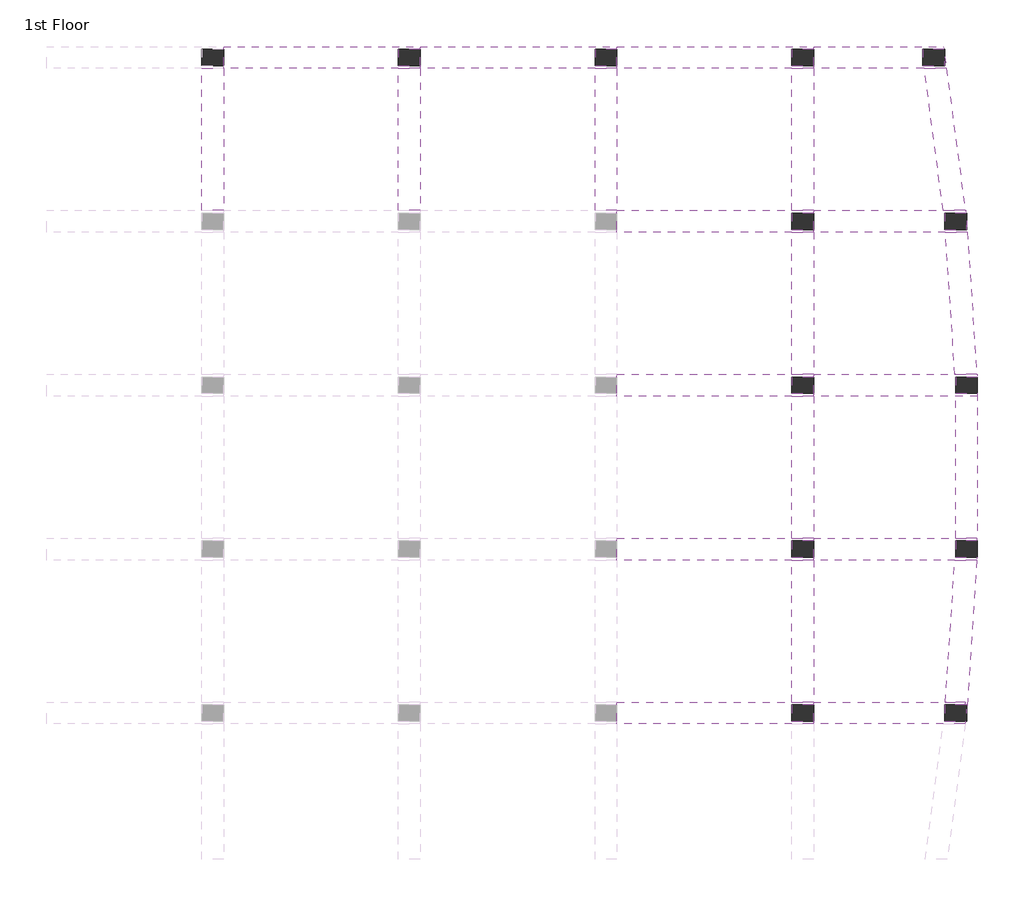
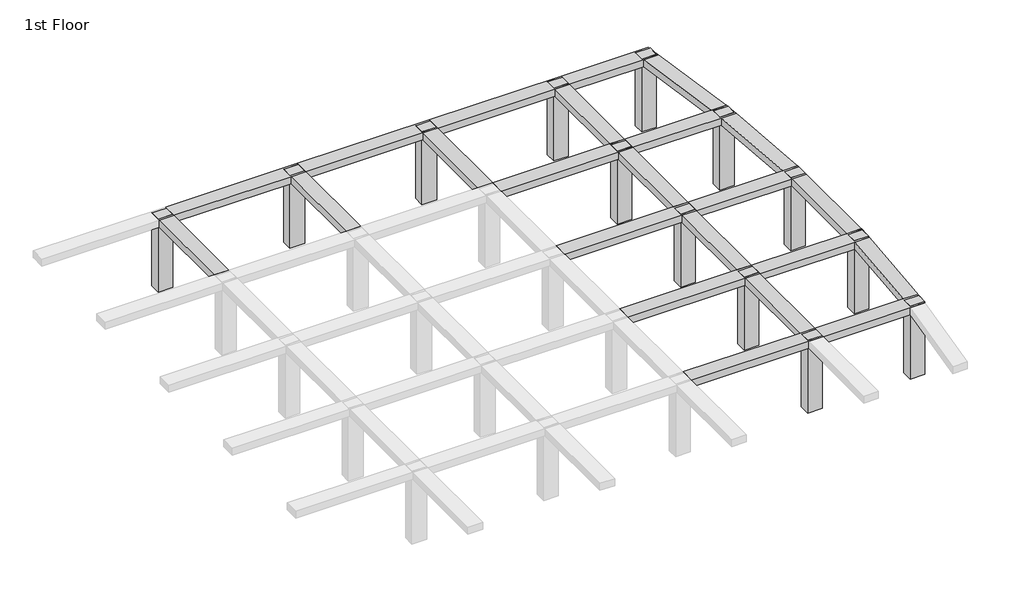
# One storey, part 3 of 3: 23 beams, 13 columns.
"""IFC4 building model written with IfcOpenShell, lengths in millimetres."""

from ifc_helpers import new_model, si_unit, frame, origin, place, context, project, spatial, polyline, outline, extrude, faceted_brep, element, save

model = new_model("IFC4")

# Units and contexts
model_context = context("Model", 3, world=origin())
ifc_project = project(units=[si_unit("LENGTHUNIT", "METRE", prefix="MILLI")], contexts=[model_context])

# Site, building, storey
site = spatial("IfcSite", under=ifc_project)
building = spatial("IfcBuilding", under=site)
storey = spatial("IfcBuildingStorey", under=building, Name="1st Floor", Elevation=3200.4)

# Beams
placement = place(None, origin())
element("IfcBeam", 1, ObjectType="Concrete-Rectangular Beam : 2' x2'", at=placement, inside=storey, context=model_context, shape_type="Brep", body=[
    faceted_brep([(-160.074232, 1680.7831222, 6400.8), (-160.074232, 1604.5831222, 6400.8), (-160.074232, 1147.3831222, 6400.8), (-160.074232, 1071.1831222, 6400.8), (4716.725768, 1071.1831222, 6400.8), (5326.325768, 1071.1831222, 6400.8), (5326.325768, 1147.3831222, 6400.8), (4716.725768, 1147.3831222, 6400.8), (4716.725768, 1604.5831222, 6400.8), (5326.325768, 1604.5831222, 6400.8), (5326.325768, 1680.7831222, 6400.8), (4716.725768, 1680.7831222, 6400.8), (-160.074232, 1071.1831222, 6096.0), (4716.725768, 1071.1831222, 6096.0), (5326.325768, 1071.1831222, 6096.0), (-160.074232, 1147.3831222, 6096.0), (-160.074232, 1604.5831222, 6096.0), (-160.074232, 1680.7831222, 6096.0), (4716.725768, 1680.7831222, 6096.0), (5326.325768, 1680.7831222, 6096.0), (5326.325768, 1604.5831222, 6096.0), (4716.725768, 1604.5831222, 6096.0), (4716.725768, 1147.3831222, 6096.0), (5326.325768, 1147.3831222, 6096.0)], [[[0, 1, 2, 3, 4, 5, 6, 7, 8, 9, 10, 11]], [[3, 12, 13, 14, 5, 4]], [[12, 15, 16, 17, 18, 19, 20, 21, 22, 23, 14, 13]], [[10, 19, 18, 17, 0, 11]], [[3, 2, 1, 0, 17, 16, 15, 12]], [[5, 14, 23, 6]], [[22, 7, 6, 23]], [[7, 22, 21, 8]], [[8, 21, 20, 9]], [[19, 10, 9, 20]]]),
])
element("IfcBeam", 2, ObjectType="Concrete-Rectangular Beam : 2' x2'", at=placement, inside=storey, context=model_context, shape_type="Brep", body=[
    faceted_brep([(9555.2251658, 1680.7831222, 6400.8), (9003.0522312, 1680.7831222, 6400.8), (5326.325768, 1680.7831222, 6400.8), (5326.325768, 1604.5831222, 6400.8), (5326.325768, 1147.3831222, 6400.8), (5326.325768, 1071.1831222, 6400.8), (8940.2370643, 1071.1831222, 6400.8), (9555.2251658, 1071.1831222, 6400.8), (9555.2251658, 1147.3831222, 6400.8), (8983.5457827, 1147.3831222, 6400.8), (8983.5457827, 1604.5831222, 6400.8), (9555.2251658, 1604.5831222, 6400.8), (9555.2251658, 1071.1831222, 6096.0), (5326.325768, 1071.1831222, 6096.0), (8940.2370643, 1071.1831222, 6096.0), (5326.325768, 1147.3831222, 6096.0), (5326.325768, 1604.5831222, 6096.0), (5326.325768, 1680.7831222, 6096.0), (9003.0522312, 1680.7831222, 6096.0), (9555.2251658, 1680.7831222, 6096.0), (9555.2251658, 1604.5831222, 6096.0), (8983.5457827, 1604.5831222, 6096.0), (8983.5457827, 1147.3831222, 6096.0), (9555.2251658, 1147.3831222, 6096.0)], [[[0, 1, 2, 3, 4, 5, 6, 7, 8, 9, 10, 11]], [[12, 7, 6, 5, 13, 14]], [[12, 14, 13, 15, 16, 17, 18, 19, 20, 21, 22, 23]], [[0, 19, 18, 17, 2, 1]], [[7, 12, 23, 8]], [[5, 4, 3, 2, 17, 16, 15, 13]], [[22, 9, 8, 23]], [[9, 22, 21, 10]], [[10, 21, 20, 11]], [[19, 0, 11, 20]]]),
])
element("IfcBeam", 3, ObjectType="Concrete-Rectangular Beam : 2' x2'", at=placement, inside=storey, context=model_context, shape_type="Brep", body=[
    faceted_brep([(-160.074232, 6252.7831222, 6400.8), (-160.074232, 6176.5831222, 6400.8), (-160.074232, 5719.3831222, 6400.8), (-160.074232, 5643.1831222, 6400.8), (4716.725768, 5643.1831222, 6400.8), (5326.325768, 5643.1831222, 6400.8), (5326.325768, 5719.3831222, 6400.8), (4716.725768, 5719.3831222, 6400.8), (4716.725768, 6176.5831222, 6400.8), (5326.325768, 6176.5831222, 6400.8), (5326.325768, 6252.7831222, 6400.8), (4716.725768, 6252.7831222, 6400.8), (-160.074232, 5643.1831222, 6096.0), (4716.725768, 5643.1831222, 6096.0), (5326.325768, 5643.1831222, 6096.0), (-160.074232, 5719.3831222, 6096.0), (-160.074232, 6176.5831222, 6096.0), (-160.074232, 6252.7831222, 6096.0), (4716.725768, 6252.7831222, 6096.0), (5326.325768, 6252.7831222, 6096.0), (5326.325768, 6176.5831222, 6096.0), (4716.725768, 6176.5831222, 6096.0), (4716.725768, 5719.3831222, 6096.0), (5326.325768, 5719.3831222, 6096.0)], [[[0, 1, 2, 3, 4, 5, 6, 7, 8, 9, 10, 11]], [[3, 12, 13, 14, 5, 4]], [[12, 15, 16, 17, 18, 19, 20, 21, 22, 23, 14, 13]], [[10, 19, 18, 17, 0, 11]], [[3, 2, 1, 0, 17, 16, 15, 12]], [[5, 14, 23, 6]], [[22, 7, 6, 23]], [[7, 22, 21, 8]], [[8, 21, 20, 9]], [[19, 10, 9, 20]]]),
])
element("IfcBeam", 4, ObjectType="Concrete-Rectangular Beam : 2' x2'", at=placement, inside=storey, context=model_context, shape_type="Brep", body=[
    faceted_brep([(9876.2389574, 6252.7831222, 6400.8), (9286.1454059, 6252.7831222, 6400.8), (5326.325768, 6252.7831222, 6400.8), (5326.325768, 6176.5831222, 6400.8), (5326.325768, 5719.3831222, 6400.8), (5326.325768, 5643.1831222, 6400.8), (9265.305238, 5643.1831222, 6400.8), (9876.2389574, 5643.1831222, 6400.8), (9876.2389574, 5719.3831222, 6400.8), (9286.1454059, 5719.3831222, 6400.8), (9286.1454059, 6176.5831222, 6400.8), (9876.2389574, 6176.5831222, 6400.8), (9876.2389574, 5643.1831222, 6096.0), (5326.325768, 5643.1831222, 6096.0), (9265.305238, 5643.1831222, 6096.0), (5326.325768, 5719.3831222, 6096.0), (5326.325768, 6176.5831222, 6096.0), (5326.325768, 6252.7831222, 6096.0), (9286.1454059, 6252.7831222, 6096.0), (9876.2389574, 6252.7831222, 6096.0), (9876.2389574, 6176.5831222, 6096.0), (9286.1454059, 6176.5831222, 6096.0), (9286.1454059, 5719.3831222, 6096.0), (9876.2389574, 5719.3831222, 6096.0)], [[[0, 1, 2, 3, 4, 5, 6, 7, 8, 9, 10, 11]], [[12, 7, 6, 5, 13, 14]], [[12, 14, 13, 15, 16, 17, 18, 19, 20, 21, 22, 23]], [[0, 19, 18, 17, 2, 1]], [[7, 12, 23, 8]], [[5, 4, 3, 2, 17, 16, 15, 13]], [[22, 9, 8, 23]], [[9, 22, 21, 10]], [[10, 21, 20, 11]], [[19, 0, 11, 20]]]),
])
element("IfcBeam", 5, ObjectType="Concrete-Rectangular Beam : 2' x2'", at=placement, inside=storey, context=model_context, shape_type="Brep", body=[
    faceted_brep([(-160.074232, 10824.7831222, 6400.8), (-160.074232, 10748.5831222, 6400.8), (-160.074232, 10291.3831222, 6400.8), (-160.074232, 10215.1831222, 6400.8), (4716.725768, 10215.1831222, 6400.8), (5326.325768, 10215.1831222, 6400.8), (5326.325768, 10291.3831222, 6400.8), (4716.725768, 10291.3831222, 6400.8), (4716.725768, 10748.5831222, 6400.8), (5326.325768, 10748.5831222, 6400.8), (5326.325768, 10824.7831222, 6400.8), (4716.725768, 10824.7831222, 6400.8), (-160.074232, 10215.1831222, 6096.0), (4716.725768, 10215.1831222, 6096.0), (5326.325768, 10215.1831222, 6096.0), (-160.074232, 10291.3831222, 6096.0), (-160.074232, 10748.5831222, 6096.0), (-160.074232, 10824.7831222, 6096.0), (4716.725768, 10824.7831222, 6096.0), (5326.325768, 10824.7831222, 6096.0), (5326.325768, 10748.5831222, 6096.0), (4716.725768, 10748.5831222, 6096.0), (4716.725768, 10291.3831222, 6096.0), (5326.325768, 10291.3831222, 6096.0)], [[[0, 1, 2, 3, 4, 5, 6, 7, 8, 9, 10, 11]], [[3, 12, 13, 14, 5, 4]], [[12, 15, 16, 17, 18, 19, 20, 21, 22, 23, 14, 13]], [[10, 19, 18, 17, 0, 11]], [[3, 2, 1, 0, 17, 16, 15, 12]], [[5, 14, 23, 6]], [[22, 7, 6, 23]], [[7, 22, 21, 8]], [[8, 21, 20, 9]], [[19, 10, 9, 20]]]),
])
element("IfcBeam", 6, ObjectType="Concrete-Rectangular Beam : 2' x2'", at=placement, inside=storey, context=model_context, shape_type="Brep", body=[
    faceted_brep([(9895.7454059, 10824.7831222, 6400.8), (9876.2389574, 10824.7831222, 6400.8), (9265.305238, 10824.7831222, 6400.8), (5326.325768, 10824.7831222, 6400.8), (5326.325768, 10748.5831222, 6400.8), (5326.325768, 10291.3831222, 6400.8), (5326.325768, 10215.1831222, 6400.8), (9895.7454059, 10215.1831222, 6400.8), (9895.7454059, 10291.3831222, 6400.8), (9286.1454059, 10291.3831222, 6400.8), (9286.1454059, 10748.5831222, 6400.8), (9895.7454059, 10748.5831222, 6400.8), (9895.7454059, 10215.1831222, 6096.0), (5326.325768, 10215.1831222, 6096.0), (5326.325768, 10291.3831222, 6096.0), (5326.325768, 10748.5831222, 6096.0), (5326.325768, 10824.7831222, 6096.0), (9265.305238, 10824.7831222, 6096.0), (9876.2389574, 10824.7831222, 6096.0), (9895.7454059, 10824.7831222, 6096.0), (9895.7454059, 10748.5831222, 6096.0), (9286.1454059, 10748.5831222, 6096.0), (9286.1454059, 10291.3831222, 6096.0), (9895.7454059, 10291.3831222, 6096.0)], [[[0, 1, 2, 3, 4, 5, 6, 7, 8, 9, 10, 11]], [[12, 7, 6, 13]], [[12, 13, 14, 15, 16, 17, 18, 19, 20, 21, 22, 23]], [[0, 19, 18, 17, 16, 3, 2, 1]], [[7, 12, 23, 8]], [[6, 5, 4, 3, 16, 15, 14, 13]], [[22, 9, 8, 23]], [[9, 22, 21, 10]], [[10, 21, 20, 11]], [[19, 0, 11, 20]]]),
])
element("IfcBeam", 7, ObjectType="Concrete-Rectangular Beam : 2' x2'", at=placement, inside=storey, context=model_context, shape_type="Brep", body=[
    faceted_brep([(-160.074232, 15396.7831222, 6400.8), (-160.074232, 15320.5831222, 6400.8), (-160.074232, 14863.3831222, 6400.8), (-160.074232, 14787.1831222, 6400.8), (4716.725768, 14787.1831222, 6400.8), (5326.325768, 14787.1831222, 6400.8), (5326.325768, 14863.3831222, 6400.8), (4716.725768, 14863.3831222, 6400.8), (4716.725768, 15320.5831222, 6400.8), (5326.325768, 15320.5831222, 6400.8), (5326.325768, 15396.7831222, 6400.8), (4716.725768, 15396.7831222, 6400.8), (-160.074232, 14787.1831222, 6096.0), (4716.725768, 14787.1831222, 6096.0), (5326.325768, 14787.1831222, 6096.0), (-160.074232, 14863.3831222, 6096.0), (-160.074232, 15320.5831222, 6096.0), (-160.074232, 15396.7831222, 6096.0), (4716.725768, 15396.7831222, 6096.0), (5326.325768, 15396.7831222, 6096.0), (5326.325768, 15320.5831222, 6096.0), (4716.725768, 15320.5831222, 6096.0), (4716.725768, 14863.3831222, 6096.0), (5326.325768, 14863.3831222, 6096.0)], [[[0, 1, 2, 3, 4, 5, 6, 7, 8, 9, 10, 11]], [[3, 12, 13, 14, 5, 4]], [[12, 15, 16, 17, 18, 19, 20, 21, 22, 23, 14, 13]], [[10, 19, 18, 17, 0, 11]], [[3, 2, 1, 0, 17, 16, 15, 12]], [[5, 14, 23, 6]], [[22, 7, 6, 23]], [[7, 22, 21, 8]], [[8, 21, 20, 9]], [[19, 10, 9, 20]]]),
])
element("IfcBeam", 8, ObjectType="Concrete-Rectangular Beam : 2' x2'", at=placement, inside=storey, context=model_context, shape_type="Brep", body=[
    faceted_brep([(9573.6393342, 15396.7831222, 6400.8), (9555.2251658, 15396.7831222, 6400.8), (8940.2370643, 15396.7831222, 6400.8), (5326.325768, 15396.7831222, 6400.8), (5326.325768, 15320.5831222, 6400.8), (5326.325768, 14863.3831222, 6400.8), (5326.325768, 14787.1831222, 6400.8), (9003.0522312, 14787.1831222, 6400.8), (9613.9859506, 14787.1831222, 6400.8), (9593.1457827, 15102.0587543, 6400.8), (9593.1457827, 14863.3831222, 6400.8), (8983.5457827, 14863.3831222, 6400.8), (8983.5457827, 15320.5831222, 6400.8), (9578.6826612, 15320.5831222, 6400.8), (9613.9859506, 14787.1831222, 6096.0), (5326.325768, 14787.1831222, 6096.0), (9003.0522312, 14787.1831222, 6096.0), (5326.325768, 14863.3831222, 6096.0), (5326.325768, 15320.5831222, 6096.0), (5326.325768, 15396.7831222, 6096.0), (8940.2370643, 15396.7831222, 6096.0), (9555.2251658, 15396.7831222, 6096.0), (9573.6393342, 15396.7831222, 6096.0), (9578.6826612, 15320.5831222, 6096.0), (8983.5457827, 15320.5831222, 6096.0), (8983.5457827, 14863.3831222, 6096.0), (9593.1457827, 14863.3831222, 6096.0), (9593.1457827, 15102.0587543, 6096.0)], [[[0, 1, 2, 3, 4, 5, 6, 7, 8, 9, 10, 11, 12, 13]], [[14, 8, 7, 6, 15, 16]], [[14, 16, 15, 17, 18, 19, 20, 21, 22, 23, 24, 25, 26, 27]], [[0, 22, 21, 20, 19, 3, 2, 1]], [[8, 14, 27, 9]], [[6, 5, 4, 3, 19, 18, 17, 15]], [[26, 10, 9, 27]], [[10, 26, 25, 11]], [[11, 25, 24, 12]], [[12, 24, 23, 13]], [[22, 0, 13, 23]]]),
])
element("IfcBeam", 9, ObjectType="Concrete-Rectangular Beam : 2' x2'", at=placement, inside=storey, context=model_context, shape_type="Brep", body=[
    faceted_brep([(-11132.874232, 19968.7831222, 6400.8), (-11132.874232, 19892.5831222, 6400.8), (-11132.874232, 19435.3831222, 6400.8), (-11132.874232, 19359.1831222, 6400.8), (-6256.074232, 19359.1831222, 6400.8), (-5646.474232, 19359.1831222, 6400.8), (-5646.474232, 19435.3831222, 6400.8), (-6256.074232, 19435.3831222, 6400.8), (-6256.074232, 19892.5831222, 6400.8), (-5646.474232, 19892.5831222, 6400.8), (-5646.474232, 19968.7831222, 6400.8), (-11132.874232, 19359.1831222, 6096.0), (-6256.074232, 19359.1831222, 6096.0), (-5646.474232, 19359.1831222, 6096.0), (-11132.874232, 19435.3831222, 6096.0), (-11132.874232, 19892.5831222, 6096.0), (-11132.874232, 19968.7831222, 6096.0), (-5646.474232, 19968.7831222, 6096.0), (-5646.474232, 19892.5831222, 6096.0), (-6256.074232, 19892.5831222, 6096.0), (-6256.074232, 19435.3831222, 6096.0), (-5646.474232, 19435.3831222, 6096.0)], [[[0, 1, 2, 3, 4, 5, 6, 7, 8, 9, 10]], [[3, 11, 12, 13, 5, 4]], [[11, 14, 15, 16, 17, 18, 19, 20, 21, 13, 12]], [[10, 17, 16, 0]], [[3, 2, 1, 0, 16, 15, 14, 11]], [[5, 13, 21, 6]], [[20, 7, 6, 21]], [[7, 20, 19, 8]], [[8, 19, 18, 9]], [[17, 10, 9, 18]]]),
])
element("IfcBeam", 10, ObjectType="Concrete-Rectangular Beam : 2' x2'", at=placement, inside=storey, context=model_context, shape_type="Brep", body=[
    faceted_brep([(-160.074232, 19968.7831222, 6400.8), (-5646.474232, 19968.7831222, 6400.8), (-5646.474232, 19892.5831222, 6400.8), (-5646.474232, 19435.3831222, 6400.8), (-5646.474232, 19359.1831222, 6400.8), (-769.674232, 19359.1831222, 6400.8), (-160.074232, 19359.1831222, 6400.8), (-160.074232, 19435.3831222, 6400.8), (-769.674232, 19435.3831222, 6400.8), (-769.674232, 19892.5831222, 6400.8), (-160.074232, 19892.5831222, 6400.8), (-160.074232, 19359.1831222, 6096.0), (-5646.474232, 19359.1831222, 6096.0), (-769.674232, 19359.1831222, 6096.0), (-5646.474232, 19435.3831222, 6096.0), (-5646.474232, 19892.5831222, 6096.0), (-5646.474232, 19968.7831222, 6096.0), (-160.074232, 19968.7831222, 6096.0), (-160.074232, 19892.5831222, 6096.0), (-769.674232, 19892.5831222, 6096.0), (-769.674232, 19435.3831222, 6096.0), (-160.074232, 19435.3831222, 6096.0)], [[[0, 1, 2, 3, 4, 5, 6, 7, 8, 9, 10]], [[11, 6, 5, 4, 12, 13]], [[11, 13, 12, 14, 15, 16, 17, 18, 19, 20, 21]], [[0, 17, 16, 1]], [[6, 11, 21, 7]], [[4, 3, 2, 1, 16, 15, 14, 12]], [[20, 8, 7, 21]], [[8, 20, 19, 9]], [[9, 19, 18, 10]], [[17, 0, 10, 18]]]),
])
element("IfcBeam", 11, ObjectType="Concrete-Rectangular Beam : 2' x2'", at=placement, inside=storey, context=model_context, shape_type="Brep", body=[
    faceted_brep([(-160.074232, 19968.7831222, 6400.8), (-160.074232, 19892.5831222, 6400.8), (-160.074232, 19435.3831222, 6400.8), (-160.074232, 19359.1831222, 6400.8), (4716.725768, 19359.1831222, 6400.8), (5326.325768, 19359.1831222, 6400.8), (5326.325768, 19435.3831222, 6400.8), (4716.725768, 19435.3831222, 6400.8), (4716.725768, 19892.5831222, 6400.8), (5326.325768, 19892.5831222, 6400.8), (5326.325768, 19968.7831222, 6400.8), (-160.074232, 19359.1831222, 6096.0), (4716.725768, 19359.1831222, 6096.0), (5326.325768, 19359.1831222, 6096.0), (-160.074232, 19435.3831222, 6096.0), (-160.074232, 19892.5831222, 6096.0), (-160.074232, 19968.7831222, 6096.0), (5326.325768, 19968.7831222, 6096.0), (5326.325768, 19892.5831222, 6096.0), (4716.725768, 19892.5831222, 6096.0), (4716.725768, 19435.3831222, 6096.0), (5326.325768, 19435.3831222, 6096.0)], [[[0, 1, 2, 3, 4, 5, 6, 7, 8, 9, 10]], [[3, 11, 12, 13, 5, 4]], [[11, 14, 15, 16, 17, 18, 19, 20, 21, 13, 12]], [[10, 17, 16, 0]], [[3, 2, 1, 0, 16, 15, 14, 11]], [[5, 13, 21, 6]], [[20, 7, 6, 21]], [[7, 20, 19, 8]], [[8, 19, 18, 9]], [[17, 10, 9, 18]]]),
])
element("IfcBeam", 12, ObjectType="Concrete-Rectangular Beam : 2' x2'", at=placement, inside=storey, context=model_context, shape_type="Brep", body=[
    faceted_brep([(5326.325768, 19968.7831222, 6400.8), (5326.325768, 19892.5831222, 6400.8), (5326.325768, 19435.3831222, 6400.8), (5326.325768, 19359.1831222, 6400.8), (8412.2463849, 19359.1831222, 6400.8), (9027.2344863, 19359.1831222, 6400.8), (8983.925768, 19684.2011052, 6400.8), (8983.925768, 19435.3831222, 6400.8), (8374.325768, 19435.3831222, 6400.8), (8374.325768, 19892.5831222, 6400.8), (8956.158818, 19892.5831222, 6400.8), (8946.005151, 19968.7831222, 6400.8), (5326.325768, 19359.1831222, 6096.0), (8412.2463849, 19359.1831222, 6096.0), (9027.2344863, 19359.1831222, 6096.0), (5326.325768, 19435.3831222, 6096.0), (5326.325768, 19892.5831222, 6096.0), (5326.325768, 19968.7831222, 6096.0), (8946.005151, 19968.7831222, 6096.0), (8956.158818, 19892.5831222, 6096.0), (8374.325768, 19892.5831222, 6096.0), (8374.325768, 19435.3831222, 6096.0), (8983.925768, 19435.3831222, 6096.0), (8983.925768, 19684.2011052, 6096.0)], [[[0, 1, 2, 3, 4, 5, 6, 7, 8, 9, 10, 11]], [[3, 12, 13, 14, 5, 4]], [[12, 15, 16, 17, 18, 19, 20, 21, 22, 23, 14, 13]], [[11, 18, 17, 0]], [[3, 2, 1, 0, 17, 16, 15, 12]], [[5, 14, 23, 6]], [[22, 7, 6, 23]], [[7, 22, 21, 8]], [[8, 21, 20, 9]], [[9, 20, 19, 10]], [[18, 11, 10, 19]]]),
])
element("IfcBeam", 13, ObjectType="Concrete-Rectangular Beam : 2' x2'", at=placement, inside=storey, context=model_context, shape_type="SweptSolid", body=[
    extrude(outline(polyline([(-11132.874232, 15396.7831222), (-11742.474232, 15396.7831222), (-11742.474232, 19359.1831222), (-11132.874232, 19359.1831222), (-11132.874232, 15396.7831222)])), frame((0.0, 0.0, 6096.0), z_axis=(0.0, 0.0, 1.0), x_axis=(1.0, 0.0, 0.0)), (0.0, 0.0, 1.0), 304.8),
])
element("IfcBeam", 14, ObjectType="Concrete-Rectangular Beam : 2' x2'", at=placement, inside=storey, context=model_context, shape_type="SweptSolid", body=[
    extrude(outline(polyline([(-5646.474232, 15396.7831222), (-6256.074232, 15396.7831222), (-6256.074232, 19359.1831222), (-5646.474232, 19359.1831222), (-5646.474232, 15396.7831222)])), frame((0.0, 0.0, 6096.0), z_axis=(0.0, 0.0, 1.0), x_axis=(1.0, 0.0, 0.0)), (0.0, 0.0, 1.0), 304.8),
])
element("IfcBeam", 15, ObjectType="Concrete-Rectangular Beam : 2' x2'", at=placement, inside=storey, context=model_context, shape_type="SweptSolid", body=[
    extrude(outline(polyline([(-160.074232, 15396.7831222), (-769.674232, 15396.7831222), (-769.674232, 19359.1831222), (-160.074232, 19359.1831222), (-160.074232, 15396.7831222)])), frame((0.0, 0.0, 6096.0), z_axis=(0.0, 0.0, 1.0), x_axis=(1.0, 0.0, 0.0)), (0.0, 0.0, 1.0), 304.8),
])
element("IfcBeam", 16, ObjectType="Concrete-Rectangular Beam : 2' x2'", at=placement, inside=storey, context=model_context, shape_type="SweptSolid", body=[
    extrude(outline(polyline([(5326.325768, 1680.7831222), (4716.725768, 1680.7831222), (4716.725768, 5643.1831222), (5326.325768, 5643.1831222), (5326.325768, 1680.7831222)])), frame((0.0, 0.0, 6096.0), z_axis=(0.0, 0.0, 1.0), x_axis=(1.0, 0.0, 0.0)), (0.0, 0.0, 1.0), 304.8),
])
element("IfcBeam", 17, ObjectType="Concrete-Rectangular Beam : 2' x2'", at=placement, inside=storey, context=model_context, shape_type="SweptSolid", body=[
    extrude(outline(polyline([(4716.725768, 10215.1831222), (5326.325768, 10215.1831222), (5326.325768, 6252.7831222), (4716.725768, 6252.7831222), (4716.725768, 10215.1831222)])), frame((0.0, 0.0, 6096.0), z_axis=(0.0, 0.0, 1.0), x_axis=(1.0, 0.0, 0.0)), (0.0, 0.0, 1.0), 304.8),
])
element("IfcBeam", 18, ObjectType="Concrete-Rectangular Beam : 2' x2'", at=placement, inside=storey, context=model_context, shape_type="SweptSolid", body=[
    extrude(outline(polyline([(4716.725768, 14787.1831222), (5326.325768, 14787.1831222), (5326.325768, 10824.7831222), (4716.725768, 10824.7831222), (4716.725768, 14787.1831222)])), frame((0.0, 0.0, 6096.0), z_axis=(0.0, 0.0, 1.0), x_axis=(1.0, 0.0, 0.0)), (0.0, 0.0, 1.0), 304.8),
])
element("IfcBeam", 19, ObjectType="Concrete-Rectangular Beam : 2' x2'", at=placement, inside=storey, context=model_context, shape_type="SweptSolid", body=[
    extrude(outline(polyline([(5326.325768, 15396.7831222), (4716.725768, 15396.7831222), (4716.725768, 19359.1831222), (5326.325768, 19359.1831222), (5326.325768, 15396.7831222)])), frame((0.0, 0.0, 6096.0), z_axis=(0.0, 0.0, 1.0), x_axis=(1.0, 0.0, 0.0)), (0.0, 0.0, 1.0), 304.8),
])
element("IfcBeam", 20, ObjectType="Concrete-Rectangular Beam : 2' x2'", at=placement, inside=storey, context=model_context, shape_type="Brep", body=[
    faceted_brep([(9916.5855738, 6252.7831222, 6400.8), (9895.7454059, 6252.7831222, 6400.8), (9876.2389574, 6252.7831222, 6400.8), (9876.2389574, 6176.5831222, 6400.8), (9895.7454059, 6176.5831222, 6400.8), (9895.7454059, 5937.9074901, 6400.8), (9916.5855738, 6252.7831222, 6096.0), (9895.7454059, 5937.9074901, 6096.0), (9876.2389574, 6252.7831222, 6096.0), (9895.7454059, 6252.7831222, 6096.0), (9895.7454059, 6176.5831222, 6096.0), (9876.2389574, 6176.5831222, 6096.0)], [[[0, 1, 2, 3, 4, 5]], [[6, 0, 5, 7]], [[8, 9, 6, 7, 10, 11]], [[0, 6, 9, 8, 2, 1]], [[4, 10, 7, 5]], [[10, 4, 3, 11]], [[2, 8, 11, 3]]]),
    faceted_brep([(9003.0522312, 1680.7831222, 6096.0), (9003.0522312, 1680.7831222, 6400.8), (9265.305238, 5643.1831222, 6400.8), (9265.305238, 5643.1831222, 6096.0), (9021.4663996, 1680.7831222, 6096.0), (9555.2251658, 1680.7831222, 6096.0), (9555.2251658, 1680.7831222, 6400.8), (9021.4663996, 1680.7831222, 6400.8), (9876.2389574, 5643.1831222, 6400.8), (9876.2389574, 5643.1831222, 6096.0), (9876.2389574, 5719.3831222, 6400.8), (9876.2389574, 5719.3831222, 6096.0), (9555.2251658, 1604.5831222, 6400.8), (9593.1457827, 1604.5831222, 6400.8), (9593.1457827, 1365.9074901, 6400.8), (9593.1457827, 1365.9074901, 6096.0), (9593.1457827, 1604.5831222, 6096.0), (9555.2251658, 1604.5831222, 6096.0), (9881.2822845, 5719.3831222, 6400.8), (9881.2822845, 5719.3831222, 6096.0)], [[[0, 1, 2, 3]], [[1, 0, 4, 5, 6, 7]], [[2, 8, 9, 3]], [[9, 8, 10, 11]], [[8, 2, 1, 7, 6, 12, 13, 14]], [[3, 9, 15, 16, 17, 5, 4, 0]], [[13, 16, 15, 14]], [[16, 13, 12, 17]], [[6, 5, 17, 12]], [[10, 18, 19, 11]], [[10, 8, 18]], [[8, 14, 15, 9, 19, 18]], [[19, 9, 11]]]),
    faceted_brep([(9555.2251658, 1071.1831222, 6400.8), (9555.2251658, 1071.1831222, 6096.0), (9565.3788327, 1147.3831222, 6096.0), (9565.3788327, 1147.3831222, 6400.8), (9555.2251658, 1147.3831222, 6400.8), (9555.2251658, 1147.3831222, 6096.0)], [[[0, 1, 2, 3]], [[1, 0, 4, 5]], [[3, 2, 5, 4]], [[4, 0, 3]], [[2, 1, 5]]]),
])
element("IfcBeam", 21, ObjectType="Concrete-Rectangular Beam : 2' x2'", at=placement, inside=storey, context=model_context, shape_type="Brep", body=[
    faceted_brep([(9895.7454059, 10824.7831222, 6400.8), (9876.2389574, 10824.7831222, 6400.8), (9286.1454059, 10824.7831222, 6400.8), (9286.1454059, 10748.5831222, 6400.8), (9895.7454059, 10748.5831222, 6400.8), (9895.7454059, 10824.7831222, 6096.0), (9895.7454059, 10748.5831222, 6096.0), (9286.1454059, 10824.7831222, 6096.0), (9876.2389574, 10824.7831222, 6096.0), (9286.1454059, 10748.5831222, 6096.0)], [[[0, 1, 2, 3, 4]], [[5, 0, 4, 6]], [[7, 8, 5, 6, 9]], [[2, 7, 9, 3]], [[2, 1, 0, 5, 8, 7]], [[4, 3, 9, 6]]]),
    faceted_brep([(9286.1454059, 6252.7831222, 6400.8), (9286.1454059, 6252.7831222, 6096.0), (9876.2389574, 6252.7831222, 6096.0), (9895.7454059, 6252.7831222, 6096.0), (9895.7454059, 6252.7831222, 6400.8), (9876.2389574, 6252.7831222, 6400.8), (9286.1454059, 10291.3831222, 6400.8), (9895.7454059, 10291.3831222, 6400.8), (9895.7454059, 10291.3831222, 6096.0), (9286.1454059, 10291.3831222, 6096.0)], [[[0, 1, 2, 3, 4, 5]], [[6, 7, 8, 9]], [[0, 5, 4, 7, 6]], [[4, 3, 8, 7]], [[3, 2, 1, 9, 8]], [[1, 0, 6, 9]]]),
])
element("IfcBeam", 22, ObjectType="Concrete-Rectangular Beam : 2' x2'", at=placement, inside=storey, context=model_context, shape_type="Brep", body=[
    faceted_brep([(9613.9859506, 14787.1831222, 6400.8), (9003.0522312, 14787.1831222, 6400.8), (9265.305238, 10824.7831222, 6400.8), (9286.1454059, 10824.7831222, 6400.8), (9876.2389574, 10824.7831222, 6400.8), (9613.9859506, 14787.1831222, 6096.0), (9876.2389574, 10824.7831222, 6096.0), (9003.0522312, 14787.1831222, 6096.0), (9286.1454059, 10824.7831222, 6096.0), (9265.305238, 10824.7831222, 6096.0)], [[[0, 1, 2, 3, 4]], [[5, 0, 4, 6]], [[7, 5, 6, 8, 9]], [[1, 7, 9, 2]], [[1, 0, 5, 7]], [[4, 3, 2, 9, 8, 6]]]),
])
element("IfcBeam", 23, ObjectType="Concrete-Rectangular Beam : 2' x2'", at=placement, inside=storey, context=model_context, shape_type="SweptSolid", body=[
    extrude(outline(polyline([(8412.2463849, 19359.1831222), (9027.2344863, 19359.1831222), (9555.2251658, 15396.7831222), (8940.2370643, 15396.7831222), (8412.2463849, 19359.1831222)])), frame((0.0, 0.0, 6096.0), z_axis=(0.0, 0.0, 1.0), x_axis=(1.0, 0.0, 0.0)), (0.0, 0.0, 1.0), 304.8),
])

# Columns
element("IfcColumn", 24, ObjectType="Concrete-Rectangular-Column : 12 x 18", at=placement, inside=storey, context=model_context, shape_type="SweptSolid", body=[
    extrude(outline(polyline([(5326.325768, 1604.5831222), (5326.325768, 1147.3831222), (4716.725768, 1147.3831222), (4716.725768, 1604.5831222), (5326.325768, 1604.5831222)])), frame((0.0, 0.0, 3200.4), z_axis=(0.0, 0.0, 1.0), x_axis=(1.0, 0.0, 0.0)), (0.0, 0.0, 1.0), 3200.4),
])
element("IfcColumn", 25, ObjectType="Concrete-Rectangular-Column : 12 x 18", at=placement, inside=storey, context=model_context, shape_type="SweptSolid", body=[
    extrude(outline(polyline([(9593.1457827, 1604.5831222), (9593.1457827, 1147.3831222), (8983.5457827, 1147.3831222), (8983.5457827, 1604.5831222), (9593.1457827, 1604.5831222)])), frame((0.0, 0.0, 3200.4), z_axis=(0.0, 0.0, 1.0), x_axis=(1.0, 0.0, 0.0)), (0.0, 0.0, 1.0), 3200.4),
])
element("IfcColumn", 26, ObjectType="Concrete-Rectangular-Column : 12 x 18", at=placement, inside=storey, context=model_context, shape_type="SweptSolid", body=[
    extrude(outline(polyline([(5326.325768, 6176.5831222), (5326.325768, 5719.3831222), (4716.725768, 5719.3831222), (4716.725768, 6176.5831222), (5326.325768, 6176.5831222)])), frame((0.0, 0.0, 3200.4), z_axis=(0.0, 0.0, 1.0), x_axis=(1.0, 0.0, 0.0)), (0.0, 0.0, 1.0), 3200.4),
])
element("IfcColumn", 27, ObjectType="Concrete-Rectangular-Column : 12 x 18", at=placement, inside=storey, context=model_context, shape_type="SweptSolid", body=[
    extrude(outline(polyline([(9895.7454059, 6176.5831222), (9895.7454059, 5719.3831222), (9286.1454059, 5719.3831222), (9286.1454059, 6176.5831222), (9895.7454059, 6176.5831222)])), frame((0.0, 0.0, 3200.4), z_axis=(0.0, 0.0, 1.0), x_axis=(1.0, 0.0, 0.0)), (0.0, 0.0, 1.0), 3200.4),
])
element("IfcColumn", 28, ObjectType="Concrete-Rectangular-Column : 12 x 18", at=placement, inside=storey, context=model_context, shape_type="SweptSolid", body=[
    extrude(outline(polyline([(5326.325768, 10748.5831222), (5326.325768, 10291.3831222), (4716.725768, 10291.3831222), (4716.725768, 10748.5831222), (5326.325768, 10748.5831222)])), frame((0.0, 0.0, 3200.4), z_axis=(0.0, 0.0, 1.0), x_axis=(1.0, 0.0, 0.0)), (0.0, 0.0, 1.0), 3200.4),
])
element("IfcColumn", 29, ObjectType="Concrete-Rectangular-Column : 12 x 18", at=placement, inside=storey, context=model_context, shape_type="SweptSolid", body=[
    extrude(outline(polyline([(9895.7454059, 10748.5831222), (9895.7454059, 10291.3831222), (9286.1454059, 10291.3831222), (9286.1454059, 10748.5831222), (9895.7454059, 10748.5831222)])), frame((0.0, 0.0, 3200.4), z_axis=(0.0, 0.0, 1.0), x_axis=(1.0, 0.0, 0.0)), (0.0, 0.0, 1.0), 3200.4),
])
element("IfcColumn", 30, ObjectType="Concrete-Rectangular-Column : 12 x 18", at=placement, inside=storey, context=model_context, shape_type="SweptSolid", body=[
    extrude(outline(polyline([(5326.325768, 15320.5831222), (5326.325768, 14863.3831222), (4716.725768, 14863.3831222), (4716.725768, 15320.5831222), (5326.325768, 15320.5831222)])), frame((0.0, 0.0, 3200.4), z_axis=(0.0, 0.0, 1.0), x_axis=(1.0, 0.0, 0.0)), (0.0, 0.0, 1.0), 3200.4),
])
element("IfcColumn", 31, ObjectType="Concrete-Rectangular-Column : 12 x 18", at=placement, inside=storey, context=model_context, shape_type="SweptSolid", body=[
    extrude(outline(polyline([(9593.1457827, 15320.5831222), (9593.1457827, 14863.3831222), (8983.5457827, 14863.3831222), (8983.5457827, 15320.5831222), (9593.1457827, 15320.5831222)])), frame((0.0, 0.0, 3200.4), z_axis=(0.0, 0.0, 1.0), x_axis=(1.0, 0.0, 0.0)), (0.0, 0.0, 1.0), 3200.4),
])
element("IfcColumn", 32, ObjectType="Concrete-Rectangular-Column : 12 x 18", at=placement, inside=storey, context=model_context, shape_type="SweptSolid", body=[
    extrude(outline(polyline([(-11132.874232, 19892.5831222), (-11132.874232, 19435.3831222), (-11742.474232, 19435.3831222), (-11742.474232, 19892.5831222), (-11132.874232, 19892.5831222)])), frame((0.0, 0.0, 3200.4), z_axis=(0.0, 0.0, 1.0), x_axis=(1.0, 0.0, 0.0)), (0.0, 0.0, 1.0), 3200.4),
])
element("IfcColumn", 33, ObjectType="Concrete-Rectangular-Column : 12 x 18", at=placement, inside=storey, context=model_context, shape_type="SweptSolid", body=[
    extrude(outline(polyline([(-5646.474232, 19892.5831222), (-5646.474232, 19435.3831222), (-6256.074232, 19435.3831222), (-6256.074232, 19892.5831222), (-5646.474232, 19892.5831222)])), frame((0.0, 0.0, 3200.4), z_axis=(0.0, 0.0, 1.0), x_axis=(1.0, 0.0, 0.0)), (0.0, 0.0, 1.0), 3200.4),
])
element("IfcColumn", 34, ObjectType="Concrete-Rectangular-Column : 12 x 18", at=placement, inside=storey, context=model_context, shape_type="SweptSolid", body=[
    extrude(outline(polyline([(-160.074232, 19892.5831222), (-160.074232, 19435.3831222), (-769.674232, 19435.3831222), (-769.674232, 19892.5831222), (-160.074232, 19892.5831222)])), frame((0.0, 0.0, 3200.4), z_axis=(0.0, 0.0, 1.0), x_axis=(1.0, 0.0, 0.0)), (0.0, 0.0, 1.0), 3200.4),
])
element("IfcColumn", 35, ObjectType="Concrete-Rectangular-Column : 12 x 18", at=placement, inside=storey, context=model_context, shape_type="SweptSolid", body=[
    extrude(outline(polyline([(5326.325768, 19892.5831222), (5326.325768, 19435.3831222), (4716.725768, 19435.3831222), (4716.725768, 19892.5831222), (5326.325768, 19892.5831222)])), frame((0.0, 0.0, 3200.4), z_axis=(0.0, 0.0, 1.0), x_axis=(1.0, 0.0, 0.0)), (0.0, 0.0, 1.0), 3200.4),
])
element("IfcColumn", 36, ObjectType="Concrete-Rectangular-Column : 12 x 18", at=placement, inside=storey, context=model_context, shape_type="SweptSolid", body=[
    extrude(outline(polyline([(8983.925768, 19892.5831222), (8983.925768, 19435.3831222), (8374.325768, 19435.3831222), (8374.325768, 19892.5831222), (8983.925768, 19892.5831222)])), frame((0.0, 0.0, 3200.4), z_axis=(0.0, 0.0, 1.0), x_axis=(1.0, 0.0, 0.0)), (0.0, 0.0, 1.0), 3200.4),
])

save(model, "model.ifc")

# Revit data of these elements
# Type "Concrete-Rectangular Beam : 2' x2'"
#   Assembly Code = "B10"
#   Length [instance default] = 5' - 0"
#   b = 2' - 0"
#   h = 1' - 0"
#   Structural Material [instance default] = Concrete, Cast-in-Place gray
# Type "Concrete-Rectangular-Column : 12 x 18"
#   Assembly Code = "B10"
#   b = 2' - 0"
#   h = 1' - 6"
#   Structural Material [instance default] = Concrete, Cast-in-Place gray
# Elements 1, 2, 3, 4, 5, 6, 7, 8, 9, 10, 11, 12, 13, 14, 15, 16, 17, 18, 19, 20, 21, 22, 23 (IfcBeam, "Concrete-Rectangular Beam : 2' x2'")
#   Structural Material = Concrete, Precast (2)
#   Phase Created = New Construction
#   Materials on its faces: "Concrete, Precast (2)"
# Elements 24, 25, 26, 27, 28, 29, 30, 31, 32, 33, 34, 35, 36 (IfcColumn, "Concrete-Rectangular-Column : 12 x 18")
#   Phase Created = New Construction
#   Materials on its faces: "Concrete, Cast-in-Place gray"
# Materials
#   "Concrete, Cast-in-Place gray": class "Concrete", colour RGB 192 192 192, transparency 0, Description = "Cast-in-place concrete", Cost = 0
#   "Concrete, Precast (2)": class "Concrete", colour RGB 198 187 187, transparency 0, Description = "Precast concrete", Cost = 0
